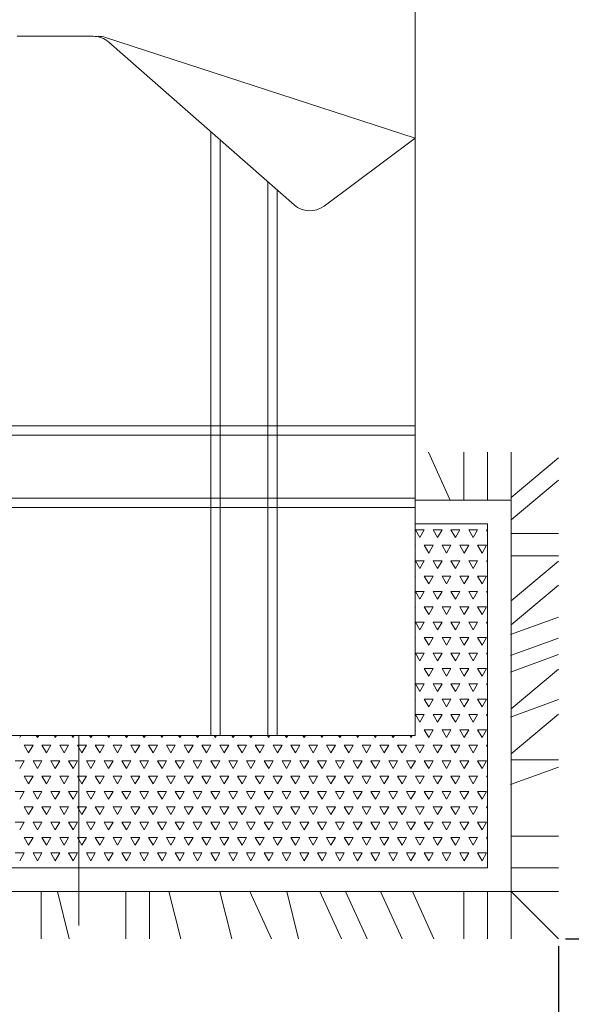
# Model space of a CAD drawing. Units: millimetres. Extents: x 225995 to 227247, y 225507 to 226008.
# Tile 20 of 23: x 227101 to 227150, y 225781 to 225868. Entities that reach past the tile are written whole.
import ezdxf

# ---------------------------------------------------------------- set-up
doc = ezdxf.new("R2010")
doc.units = ezdxf.units.MM
for name, color, linetype, lineweight in [('A-ANNO-DIMS', 2, 'Continuous', 18), ('A-FLOR-PATT', 8, 'Continuous', 13), ('A-FURN', 9, 'Continuous', 18)]:
    doc.layers.add(name, color=color, linetype=linetype, lineweight=lineweight)
doc.styles.get("Standard").update_dxf_attribs({"font": 'arial.ttf'})
doc.dimstyles.new('ISO-25', dxfattribs={"dimtxt": 6, "dimasz": 2.5, "dimexe": 1.25, "dimexo": 0.625, "dimtad": 1, "dimdec": 0, "dimlunit": 3, "dimtxsty": 'Standard', "dimcen": 2.5, "dimadec": 0, "dimazin": 0, "dimtfac": 1, "dimtdec": 0, "dimtmove": 0, "dimatfit": 3, "dimfxl": 1, "dimarcsym": 0})

# ---------------------------------------------------------------- blocks, each defined once
blk = doc.blocks.new('A$C6D2A2628')
for p, q in [((1.791, 2.4297), (1.791, 0.4297)), ((0.9515, 1.9058), (1.1116, 1.9058)), ((1.791, 1.6908), (1.138, 1.9034)), ((1.1446, 1.8934), (1.5358, 1.5497)), ((1.3599, 1.7043), (1.3599, 0.4297)), ((1.3799, 1.6867), (1.3799, 0.4297)), ((1.5987, 1.5472), (1.791, 1.6908)), ((1.4799, 1.5988), (1.4799, 0.4297)), ((1.4999, 1.5812), (1.4999, 0.4297)), ((0.291, 1.0837), (1.791, 1.0837)), ((0.291, 1.0637), (1.791, 1.0637)), ((1.8187, 1.0278), (1.8641, 0.9278)), ((1.8932, 1.0278), (1.8932, 0.9278)), ((1.9432, 1.0278), (1.9432, 0.9278)), ((1.9932, 1.0278), (1.9932, 0.9278)), ((1.9932, 0.9324), (2.0932, 1.016)), ((1.9932, 0.8849), (2.0932, 0.9685)), ((0.291, 0.9307), (1.791, 0.9307)), ((1.9932, 0.9267), (1.791, 0.9267)), ((1.9932, 0.1), (1.9932, 0.9267)), ((0.291, 0.9107), (1.791, 0.9107)), ((1.9432, 0.8767), (1.791, 0.8767)), ((1.9432, 0.15), (1.9432, 0.8767)), ((1.8007, 0.8473), (1.7913, 0.8636)), ((1.7913, 0.8636), (1.8101, 0.8636)), ((1.8007, 0.8473), (1.8101, 0.8636)), ((1.8382, 0.8473), (1.8288, 0.8636)), ((1.8288, 0.8636), (1.8476, 0.8636)), ((1.8382, 0.8473), (1.8476, 0.8636)), ((1.8757, 0.8473), (1.8663, 0.8636)), ((1.8663, 0.8636), (1.8851, 0.8636)), ((1.8757, 0.8473), (1.8851, 0.8636)), ((1.9132, 0.8473), (1.9038, 0.8636)), ((1.9038, 0.8636), (1.9226, 0.8636)), ((1.9132, 0.8473), (1.9226, 0.8636)), ((1.9432, 0.8604), (1.9413, 0.8636)), ((1.9413, 0.8636), (1.9432, 0.8636)), ((1.9932, 0.8564), (2.0932, 0.8564)), ((1.791, 0.8305), (1.7913, 0.8311)), ((1.791, 0.8311), (1.7913, 0.8311)), ((1.8195, 0.8148), (1.8101, 0.8311)), ((1.8101, 0.8311), (1.8288, 0.8311)), ((1.8195, 0.8148), (1.8288, 0.8311)), ((1.857, 0.8148), (1.8476, 0.8311)), ((1.8476, 0.8311), (1.8663, 0.8311)), ((1.857, 0.8148), (1.8663, 0.8311)), ((1.8945, 0.8148), (1.8851, 0.8311)), ((1.8851, 0.8311), (1.9038, 0.8311)), ((1.8945, 0.8148), (1.9038, 0.8311)), ((1.932, 0.8148), (1.9226, 0.8311)), ((1.9226, 0.8311), (1.9413, 0.8311)), ((1.932, 0.8148), (1.9413, 0.8311)), ((1.8007, 0.7824), (1.7913, 0.7986)), ((1.7913, 0.7986), (1.8101, 0.7986)), ((1.8007, 0.7824), (1.8101, 0.7986)), ((1.8382, 0.7824), (1.8288, 0.7986)), ((1.8288, 0.7986), (1.8476, 0.7986)), ((1.8382, 0.7824), (1.8476, 0.7986)), ((1.8757, 0.7824), (1.8663, 0.7986)), ((1.8663, 0.7986), (1.8851, 0.7986)), ((1.8757, 0.7824), (1.8851, 0.7986)), ((1.9132, 0.7824), (1.9038, 0.7986)), ((1.9038, 0.7986), (1.9226, 0.7986)), ((1.9132, 0.7824), (1.9226, 0.7986)), ((1.9432, 0.7955), (1.9413, 0.7986)), ((1.9413, 0.7986), (1.9432, 0.7986)), ((1.9932, 0.8089), (2.0932, 0.8089)), ((1.9932, 0.7139), (2.0932, 0.7975)), ((1.791, 0.7655), (1.7913, 0.7661)), ((1.791, 0.7661), (1.7913, 0.7661)), ((1.8195, 0.7499), (1.8101, 0.7661)), ((1.8101, 0.7661), (1.8288, 0.7661)), ((1.8195, 0.7499), (1.8288, 0.7661)), ((1.857, 0.7499), (1.8476, 0.7661)), ((1.8476, 0.7661), (1.8663, 0.7661)), ((1.857, 0.7499), (1.8663, 0.7661)), ((1.8945, 0.7499), (1.8851, 0.7661)), ((1.8851, 0.7661), (1.9038, 0.7661)), ((1.8945, 0.7499), (1.9038, 0.7661)), ((1.932, 0.7499), (1.9226, 0.7661)), ((1.9226, 0.7661), (1.9413, 0.7661)), ((1.932, 0.7499), (1.9413, 0.7661)), ((1.8007, 0.7174), (1.7913, 0.7337)), ((1.7913, 0.7337), (1.8101, 0.7337)), ((1.8007, 0.7174), (1.8101, 0.7337)), ((1.8382, 0.7174), (1.8288, 0.7337)), ((1.8288, 0.7337), (1.8476, 0.7337)), ((1.8382, 0.7174), (1.8476, 0.7337)), ((1.8757, 0.7174), (1.8663, 0.7337)), ((1.8663, 0.7337), (1.8851, 0.7337)), ((1.8757, 0.7174), (1.8851, 0.7337)), ((1.9132, 0.7174), (1.9038, 0.7337)), ((1.9038, 0.7337), (1.9226, 0.7337)), ((1.9132, 0.7174), (1.9226, 0.7337)), ((1.9432, 0.7305), (1.9413, 0.7337)), ((1.9413, 0.7337), (1.9432, 0.7337)), ((1.9932, 0.6633), (2.0932, 0.7469)), ((1.791, 0.7006), (1.7913, 0.7012)), ((1.791, 0.7012), (1.7913, 0.7012)), ((1.8195, 0.6849), (1.8101, 0.7012)), ((1.8101, 0.7012), (1.8288, 0.7012)), ((1.8195, 0.6849), (1.8288, 0.7012)), ((1.857, 0.6849), (1.8476, 0.7012)), ((1.8476, 0.7012), (1.8663, 0.7012)), ((1.857, 0.6849), (1.8663, 0.7012)), ((1.8945, 0.6849), (1.8851, 0.7012)), ((1.8851, 0.7012), (1.9038, 0.7012)), ((1.8945, 0.6849), (1.9038, 0.7012)), ((1.932, 0.6849), (1.9226, 0.7012)), ((1.9226, 0.7012), (1.9413, 0.7012)), ((1.932, 0.6849), (1.9413, 0.7012)), ((1.8007, 0.6525), (1.7913, 0.6687)), ((1.7913, 0.6687), (1.8101, 0.6687)), ((1.8007, 0.6525), (1.8101, 0.6687)), ((1.8382, 0.6525), (1.8288, 0.6687)), ((1.8288, 0.6687), (1.8476, 0.6687)), ((1.8382, 0.6525), (1.8476, 0.6687)), ((1.8757, 0.6525), (1.8663, 0.6687)), ((1.8663, 0.6687), (1.8851, 0.6687)), ((1.8757, 0.6525), (1.8851, 0.6687)), ((1.9132, 0.6525), (1.9038, 0.6687)), ((1.9038, 0.6687), (1.9226, 0.6687)), ((1.9132, 0.6525), (1.9226, 0.6687)), ((1.9432, 0.6655), (1.9413, 0.6687)), ((1.9413, 0.6687), (1.9432, 0.6687)), ((1.9917, 0.6428), (2.0932, 0.6794)), ((1.791, 0.6356), (1.7913, 0.6362)), ((1.791, 0.6362), (1.7913, 0.6362)), ((1.8195, 0.62), (1.8101, 0.6362)), ((1.8101, 0.6362), (1.8288, 0.6362)), ((1.8195, 0.62), (1.8288, 0.6362)), ((1.857, 0.62), (1.8476, 0.6362)), ((1.8476, 0.6362), (1.8663, 0.6362)), ((1.857, 0.62), (1.8663, 0.6362)), ((1.8945, 0.62), (1.8851, 0.6362)), ((1.8851, 0.6362), (1.9038, 0.6362)), ((1.8945, 0.62), (1.9038, 0.6362)), ((1.932, 0.62), (1.9226, 0.6362)), ((1.9226, 0.6362), (1.9413, 0.6362)), ((1.932, 0.62), (1.9413, 0.6362)), ((1.9917, 0.5984), (2.0932, 0.6351)), ((1.8007, 0.5875), (1.7913, 0.6037)), ((1.7913, 0.6037), (1.8101, 0.6037)), ((1.8007, 0.5875), (1.8101, 0.6037)), ((1.8382, 0.5875), (1.8288, 0.6037)), ((1.8288, 0.6037), (1.8476, 0.6037)), ((1.8382, 0.5875), (1.8476, 0.6037)), ((1.8757, 0.5875), (1.8663, 0.6037)), ((1.8663, 0.6037), (1.8851, 0.6037)), ((1.8757, 0.5875), (1.8851, 0.6037)), ((1.9132, 0.5875), (1.9038, 0.6037)), ((1.9038, 0.6037), (1.9226, 0.6037)), ((1.9132, 0.5875), (1.9226, 0.6037)), ((1.9432, 0.6006), (1.9413, 0.6037)), ((1.9413, 0.6037), (1.9432, 0.6037)), ((1.9917, 0.5636), (2.0932, 0.6003)), ((1.791, 0.5707), (1.7913, 0.5713)), ((1.791, 0.5713), (1.7913, 0.5713)), ((1.8195, 0.555), (1.8101, 0.5713)), ((1.8101, 0.5713), (1.8288, 0.5713)), ((1.8195, 0.555), (1.8288, 0.5713)), ((1.857, 0.555), (1.8476, 0.5713)), ((1.8476, 0.5713), (1.8663, 0.5713)), ((1.857, 0.555), (1.8663, 0.5713)), ((1.8945, 0.555), (1.8851, 0.5713)), ((1.8851, 0.5713), (1.9038, 0.5713)), ((1.8945, 0.555), (1.9038, 0.5713)), ((1.932, 0.555), (1.9226, 0.5713)), ((1.9226, 0.5713), (1.9413, 0.5713)), ((1.932, 0.555), (1.9413, 0.5713)), ((1.9932, 0.4859), (2.0932, 0.5695)), ((1.8007, 0.5226), (1.7913, 0.5388)), ((1.7913, 0.5388), (1.8101, 0.5388)), ((1.8007, 0.5226), (1.8101, 0.5388)), ((1.8382, 0.5226), (1.8288, 0.5388)), ((1.8288, 0.5388), (1.8476, 0.5388)), ((1.8382, 0.5226), (1.8476, 0.5388)), ((1.8757, 0.5226), (1.8663, 0.5388)), ((1.8663, 0.5388), (1.8851, 0.5388)), ((1.8757, 0.5226), (1.8851, 0.5388)), ((1.9132, 0.5226), (1.9038, 0.5388)), ((1.9038, 0.5388), (1.9226, 0.5388)), ((1.9132, 0.5226), (1.9226, 0.5388)), ((1.9432, 0.5356), (1.9413, 0.5388)), ((1.9413, 0.5388), (1.9432, 0.5388)), ((1.791, 0.5057), (1.7913, 0.5063)), ((1.791, 0.5063), (1.7913, 0.5063)), ((1.8195, 0.4901), (1.8101, 0.5063)), ((1.8101, 0.5063), (1.8288, 0.5063)), ((1.8195, 0.4901), (1.8288, 0.5063)), ((1.857, 0.4901), (1.8476, 0.5063)), ((1.8476, 0.5063), (1.8663, 0.5063)), ((1.857, 0.4901), (1.8663, 0.5063)), ((1.8945, 0.4901), (1.8851, 0.5063)), ((1.8851, 0.5063), (1.9038, 0.5063)), ((1.8945, 0.4901), (1.9038, 0.5063)), ((1.932, 0.4901), (1.9226, 0.5063)), ((1.9226, 0.5063), (1.9413, 0.5063)), ((1.932, 0.4901), (1.9413, 0.5063)), ((1.9917, 0.4686), (2.0932, 0.5053)), ((1.8007, 0.4576), (1.7913, 0.4738)), ((1.7913, 0.4738), (1.8101, 0.4738)), ((1.8007, 0.4576), (1.8101, 0.4738)), ((1.8382, 0.4576), (1.8288, 0.4738)), ((1.8288, 0.4738), (1.8476, 0.4738)), ((1.8382, 0.4576), (1.8476, 0.4738)), ((1.8757, 0.4576), (1.8663, 0.4738)), ((1.8663, 0.4738), (1.8851, 0.4738)), ((1.8757, 0.4576), (1.8851, 0.4738)), ((1.9132, 0.4576), (1.9038, 0.4738)), ((1.9038, 0.4738), (1.9226, 0.4738)), ((1.9132, 0.4576), (1.9226, 0.4738)), ((1.9432, 0.4707), (1.9413, 0.4738)), ((1.9413, 0.4738), (1.9432, 0.4738)), ((1.9932, 0.3909), (2.0932, 0.4745)), ((1.791, 0.4408), (1.7913, 0.4414)), ((1.791, 0.4414), (1.7913, 0.4414)), ((1.8195, 0.4251), (1.8101, 0.4414)), ((1.8101, 0.4414), (1.8288, 0.4414)), ((1.8195, 0.4251), (1.8288, 0.4414)), ((1.857, 0.4251), (1.8476, 0.4414)), ((1.8476, 0.4414), (1.8663, 0.4414)), ((1.857, 0.4251), (1.8663, 0.4414)), ((1.8945, 0.4251), (1.8851, 0.4414)), ((1.8851, 0.4414), (1.9038, 0.4414)), ((1.8945, 0.4251), (1.9038, 0.4414)), ((1.932, 0.4251), (1.9226, 0.4414)), ((1.9226, 0.4414), (1.9413, 0.4414)), ((1.932, 0.4251), (1.9413, 0.4414)), ((1.791, 0.4297), (0.291, 0.4297)), ((0.957, 0.4251), (0.9596, 0.4297)), ((0.9945, 0.4251), (0.9918, 0.4297)), ((0.9945, 0.4251), (0.9971, 0.4297)), ((1.032, 0.4251), (1.0293, 0.4297)), ((1.032, 0.4251), (1.0346, 0.4297)), ((1.0695, 0.4251), (1.0668, 0.4297)), ((1.0695, 0.4251), (1.0721, 0.4297)), ((1.107, 0.4251), (1.1043, 0.4297)), ((1.107, 0.4251), (1.1096, 0.4297)), ((1.1445, 0.4251), (1.1418, 0.4297)), ((1.1445, 0.4251), (1.1471, 0.4297)), ((1.182, 0.4251), (1.1793, 0.4297)), ((1.182, 0.4251), (1.1846, 0.4297)), ((1.2195, 0.4251), (1.2168, 0.4297)), ((1.2195, 0.4251), (1.2221, 0.4297)), ((1.257, 0.4251), (1.2543, 0.4297)), ((1.257, 0.4251), (1.2596, 0.4297)), ((1.2945, 0.4251), (1.2918, 0.4297)), ((1.2945, 0.4251), (1.2971, 0.4297)), ((1.332, 0.4251), (1.3293, 0.4297)), ((1.332, 0.4251), (1.3346, 0.4297)), ((1.3695, 0.4251), (1.3668, 0.4297)), ((1.3695, 0.4251), (1.3721, 0.4297)), ((1.407, 0.4251), (1.4043, 0.4297)), ((1.407, 0.4251), (1.4096, 0.4297)), ((1.4445, 0.4251), (1.4418, 0.4297)), ((1.4445, 0.4251), (1.4471, 0.4297)), ((1.482, 0.4251), (1.4793, 0.4297)), ((1.482, 0.4251), (1.4846, 0.4297)), ((1.5195, 0.4251), (1.5168, 0.4297)), ((1.5195, 0.4251), (1.5221, 0.4297)), ((1.557, 0.4251), (1.5543, 0.4297)), ((1.557, 0.4251), (1.5596, 0.4297)), ((1.5945, 0.4251), (1.5918, 0.4297)), ((1.5945, 0.4251), (1.5971, 0.4297)), ((1.632, 0.4251), (1.6293, 0.4297)), ((1.632, 0.4251), (1.6346, 0.4297)), ((1.6695, 0.4251), (1.6668, 0.4297)), ((1.6695, 0.4251), (1.6721, 0.4297)), ((1.707, 0.4251), (1.7043, 0.4297)), ((1.707, 0.4251), (1.7096, 0.4297)), ((1.7445, 0.4251), (1.7418, 0.4297)), ((1.7445, 0.4251), (1.7471, 0.4297)), ((1.782, 0.4251), (1.7793, 0.4297)), ((1.782, 0.4251), (1.7846, 0.4297)), ((0.9757, 0.3927), (0.9663, 0.4089)), ((0.9663, 0.4089), (0.9851, 0.4089)), ((0.9757, 0.3927), (0.9851, 0.4089)), ((1.0132, 0.3927), (1.0038, 0.4089)), ((1.0038, 0.4089), (1.0226, 0.4089)), ((1.0132, 0.3927), (1.0226, 0.4089)), ((1.0507, 0.3927), (1.0413, 0.4089)), ((1.0413, 0.4089), (1.0601, 0.4089)), ((1.0507, 0.3927), (1.0601, 0.4089)), ((1.0882, 0.3927), (1.0788, 0.4089)), ((1.0788, 0.4089), (1.0976, 0.4089)), ((1.0882, 0.3927), (1.0976, 0.4089)), ((1.1257, 0.3927), (1.1163, 0.4089)), ((1.1163, 0.4089), (1.1351, 0.4089)), ((1.1257, 0.3927), (1.1351, 0.4089)), ((1.1632, 0.3927), (1.1538, 0.4089)), ((1.1538, 0.4089), (1.1726, 0.4089)), ((1.1632, 0.3927), (1.1726, 0.4089)), ((1.2007, 0.3927), (1.1913, 0.4089)), ((1.1913, 0.4089), (1.2101, 0.4089)), ((1.2007, 0.3927), (1.2101, 0.4089)), ((1.2382, 0.3927), (1.2288, 0.4089)), ((1.2288, 0.4089), (1.2476, 0.4089)), ((1.2382, 0.3927), (1.2476, 0.4089)), ((1.2757, 0.3927), (1.2663, 0.4089)), ((1.2663, 0.4089), (1.2851, 0.4089)), ((1.2757, 0.3927), (1.2851, 0.4089)), ((1.3132, 0.3927), (1.3038, 0.4089)), ((1.3038, 0.4089), (1.3226, 0.4089)), ((1.3132, 0.3927), (1.3226, 0.4089)), ((1.3507, 0.3927), (1.3413, 0.4089)), ((1.3413, 0.4089), (1.3601, 0.4089)), ((1.3507, 0.3927), (1.3601, 0.4089)), ((1.3882, 0.3927), (1.3788, 0.4089)), ((1.3788, 0.4089), (1.3976, 0.4089)), ((1.3882, 0.3927), (1.3976, 0.4089)), ((1.4257, 0.3927), (1.4163, 0.4089)), ((1.4163, 0.4089), (1.4351, 0.4089)), ((1.4257, 0.3927), (1.4351, 0.4089)), ((1.4632, 0.3927), (1.4538, 0.4089)), ((1.4538, 0.4089), (1.4726, 0.4089)), ((1.4632, 0.3927), (1.4726, 0.4089)), ((1.5007, 0.3927), (1.4913, 0.4089)), ((1.4913, 0.4089), (1.5101, 0.4089)), ((1.5007, 0.3927), (1.5101, 0.4089)), ((1.5382, 0.3927), (1.5288, 0.4089)), ((1.5288, 0.4089), (1.5476, 0.4089)), ((1.5382, 0.3927), (1.5476, 0.4089)), ((1.5757, 0.3927), (1.5663, 0.4089)), ((1.5663, 0.4089), (1.5851, 0.4089)), ((1.5757, 0.3927), (1.5851, 0.4089)), ((1.6132, 0.3927), (1.6038, 0.4089)), ((1.6038, 0.4089), (1.6226, 0.4089)), ((1.6132, 0.3927), (1.6226, 0.4089)), ((1.6507, 0.3927), (1.6413, 0.4089)), ((1.6413, 0.4089), (1.6601, 0.4089)), ((1.6507, 0.3927), (1.6601, 0.4089)), ((1.6882, 0.3927), (1.6788, 0.4089)), ((1.6788, 0.4089), (1.6976, 0.4089)), ((1.6882, 0.3927), (1.6976, 0.4089)), ((1.7257, 0.3927), (1.7163, 0.4089)), ((1.7163, 0.4089), (1.7351, 0.4089)), ((1.7257, 0.3927), (1.7351, 0.4089)), ((1.7632, 0.3927), (1.7538, 0.4089)), ((1.7538, 0.4089), (1.7726, 0.4089)), ((1.7632, 0.3927), (1.7726, 0.4089)), ((1.8007, 0.3927), (1.7913, 0.4089)), ((1.7913, 0.4089), (1.8101, 0.4089)), ((1.8007, 0.3927), (1.8101, 0.4089)), ((1.8382, 0.3927), (1.8288, 0.4089)), ((1.8288, 0.4089), (1.8476, 0.4089)), ((1.8382, 0.3927), (1.8476, 0.4089)), ((1.8757, 0.3927), (1.8663, 0.4089)), ((1.8663, 0.4089), (1.8851, 0.4089)), ((1.8757, 0.3927), (1.8851, 0.4089)), ((1.9132, 0.3927), (1.9038, 0.4089)), ((1.9038, 0.4089), (1.9226, 0.4089)), ((1.9132, 0.3927), (1.9226, 0.4089)), ((1.9432, 0.4057), (1.9413, 0.4089)), ((1.9413, 0.4089), (1.9432, 0.4089)), ((0.9476, 0.3764), (0.9663, 0.3764)), ((0.957, 0.3602), (0.9663, 0.3764)), ((0.9945, 0.3602), (0.9851, 0.3764)), ((0.9851, 0.3764), (1.0038, 0.3764)), ((0.9945, 0.3602), (1.0038, 0.3764)), ((1.032, 0.3602), (1.0226, 0.3764)), ((1.0226, 0.3764), (1.0413, 0.3764)), ((1.032, 0.3602), (1.0413, 0.3764)), ((1.0695, 0.3602), (1.0601, 0.3764)), ((1.0601, 0.3764), (1.0788, 0.3764)), ((1.0695, 0.3602), (1.0788, 0.3764)), ((1.107, 0.3602), (1.0976, 0.3764)), ((1.0976, 0.3764), (1.1163, 0.3764)), ((1.107, 0.3602), (1.1163, 0.3764)), ((1.1445, 0.3602), (1.1351, 0.3764)), ((1.1351, 0.3764), (1.1538, 0.3764)), ((1.1445, 0.3602), (1.1538, 0.3764)), ((1.182, 0.3602), (1.1726, 0.3764)), ((1.1726, 0.3764), (1.1913, 0.3764)), ((1.182, 0.3602), (1.1913, 0.3764)), ((1.2195, 0.3602), (1.2101, 0.3764)), ((1.2101, 0.3764), (1.2288, 0.3764)), ((1.2195, 0.3602), (1.2288, 0.3764)), ((1.257, 0.3602), (1.2476, 0.3764)), ((1.2476, 0.3764), (1.2663, 0.3764)), ((1.257, 0.3602), (1.2663, 0.3764)), ((1.2945, 0.3602), (1.2851, 0.3764)), ((1.2851, 0.3764), (1.3038, 0.3764)), ((1.2945, 0.3602), (1.3038, 0.3764)), ((1.332, 0.3602), (1.3226, 0.3764)), ((1.3226, 0.3764), (1.3413, 0.3764)), ((1.332, 0.3602), (1.3413, 0.3764)), ((1.3695, 0.3602), (1.3601, 0.3764)), ((1.3601, 0.3764), (1.3788, 0.3764)), ((1.3695, 0.3602), (1.3788, 0.3764)), ((1.407, 0.3602), (1.3976, 0.3764)), ((1.3976, 0.3764), (1.4163, 0.3764)), ((1.407, 0.3602), (1.4163, 0.3764)), ((1.4445, 0.3602), (1.4351, 0.3764)), ((1.4351, 0.3764), (1.4538, 0.3764)), ((1.4445, 0.3602), (1.4538, 0.3764)), ((1.482, 0.3602), (1.4726, 0.3764)), ((1.4726, 0.3764), (1.4913, 0.3764)), ((1.482, 0.3602), (1.4913, 0.3764)), ((1.5195, 0.3602), (1.5101, 0.3764)), ((1.5101, 0.3764), (1.5288, 0.3764)), ((1.5195, 0.3602), (1.5288, 0.3764)), ((1.557, 0.3602), (1.5476, 0.3764)), ((1.5476, 0.3764), (1.5663, 0.3764)), ((1.557, 0.3602), (1.5663, 0.3764)), ((1.5945, 0.3602), (1.5851, 0.3764)), ((1.5851, 0.3764), (1.6038, 0.3764)), ((1.5945, 0.3602), (1.6038, 0.3764)), ((1.632, 0.3602), (1.6226, 0.3764)), ((1.6226, 0.3764), (1.6413, 0.3764)), ((1.632, 0.3602), (1.6413, 0.3764)), ((1.6695, 0.3602), (1.6601, 0.3764)), ((1.6601, 0.3764), (1.6788, 0.3764)), ((1.6695, 0.3602), (1.6788, 0.3764)), ((1.707, 0.3602), (1.6976, 0.3764)), ((1.6976, 0.3764), (1.7163, 0.3764)), ((1.707, 0.3602), (1.7163, 0.3764)), ((1.7445, 0.3602), (1.7351, 0.3764)), ((1.7351, 0.3764), (1.7538, 0.3764)), ((1.7445, 0.3602), (1.7538, 0.3764)), ((1.782, 0.3602), (1.7726, 0.3764)), ((1.7726, 0.3764), (1.7913, 0.3764)), ((1.782, 0.3602), (1.7913, 0.3764)), ((1.8195, 0.3602), (1.8101, 0.3764)), ((1.8101, 0.3764), (1.8288, 0.3764)), ((1.8195, 0.3602), (1.8288, 0.3764)), ((1.857, 0.3602), (1.8476, 0.3764)), ((1.8476, 0.3764), (1.8663, 0.3764)), ((1.857, 0.3602), (1.8663, 0.3764)), ((1.8945, 0.3602), (1.8851, 0.3764)), ((1.8851, 0.3764), (1.9038, 0.3764)), ((1.8945, 0.3602), (1.9038, 0.3764)), ((1.932, 0.3602), (1.9226, 0.3764)), ((1.9226, 0.3764), (1.9413, 0.3764)), ((1.932, 0.3602), (1.9413, 0.3764)), ((1.9932, 0.3783), (2.0932, 0.3783)), ((1.9917, 0.3261), (2.0932, 0.3628)), ((0.9757, 0.3277), (0.9663, 0.3439)), ((0.9663, 0.3439), (0.9851, 0.3439)), ((0.9757, 0.3277), (0.9851, 0.3439)), ((1.0132, 0.3277), (1.0038, 0.3439)), ((1.0038, 0.3439), (1.0226, 0.3439)), ((1.0132, 0.3277), (1.0226, 0.3439)), ((1.0507, 0.3277), (1.0413, 0.3439)), ((1.0413, 0.3439), (1.0601, 0.3439)), ((1.0507, 0.3277), (1.0601, 0.3439)), ((1.0882, 0.3277), (1.0788, 0.3439)), ((1.0788, 0.3439), (1.0976, 0.3439)), ((1.0882, 0.3277), (1.0976, 0.3439)), ((1.1257, 0.3277), (1.1163, 0.3439)), ((1.1163, 0.3439), (1.1351, 0.3439)), ((1.1257, 0.3277), (1.1351, 0.3439)), ((1.1632, 0.3277), (1.1538, 0.3439)), ((1.1538, 0.3439), (1.1726, 0.3439)), ((1.1632, 0.3277), (1.1726, 0.3439)), ((1.2007, 0.3277), (1.1913, 0.3439)), ((1.1913, 0.3439), (1.2101, 0.3439)), ((1.2007, 0.3277), (1.2101, 0.3439)), ((1.2382, 0.3277), (1.2288, 0.3439)), ((1.2288, 0.3439), (1.2476, 0.3439)), ((1.2382, 0.3277), (1.2476, 0.3439)), ((1.2757, 0.3277), (1.2663, 0.3439)), ((1.2663, 0.3439), (1.2851, 0.3439)), ((1.2757, 0.3277), (1.2851, 0.3439)), ((1.3132, 0.3277), (1.3038, 0.3439)), ((1.3038, 0.3439), (1.3226, 0.3439)), ((1.3132, 0.3277), (1.3226, 0.3439)), ((1.3507, 0.3277), (1.3413, 0.3439)), ((1.3413, 0.3439), (1.3601, 0.3439)), ((1.3507, 0.3277), (1.3601, 0.3439)), ((1.3882, 0.3277), (1.3788, 0.3439)), ((1.3788, 0.3439), (1.3976, 0.3439)), ((1.3882, 0.3277), (1.3976, 0.3439)), ((1.4257, 0.3277), (1.4163, 0.3439)), ((1.4163, 0.3439), (1.4351, 0.3439)), ((1.4257, 0.3277), (1.4351, 0.3439)), ((1.4632, 0.3277), (1.4538, 0.3439)), ((1.4538, 0.3439), (1.4726, 0.3439)), ((1.4632, 0.3277), (1.4726, 0.3439)), ((1.5007, 0.3277), (1.4913, 0.3439)), ((1.4913, 0.3439), (1.5101, 0.3439)), ((1.5007, 0.3277), (1.5101, 0.3439)), ((1.5382, 0.3277), (1.5288, 0.3439)), ((1.5288, 0.3439), (1.5476, 0.3439)), ((1.5382, 0.3277), (1.5476, 0.3439)), ((1.5757, 0.3277), (1.5663, 0.3439)), ((1.5663, 0.3439), (1.5851, 0.3439)), ((1.5757, 0.3277), (1.5851, 0.3439)), ((1.6132, 0.3277), (1.6038, 0.3439)), ((1.6038, 0.3439), (1.6226, 0.3439)), ((1.6132, 0.3277), (1.6226, 0.3439)), ((1.6507, 0.3277), (1.6413, 0.3439)), ((1.6413, 0.3439), (1.6601, 0.3439)), ((1.6507, 0.3277), (1.6601, 0.3439)), ((1.6882, 0.3277), (1.6788, 0.3439)), ((1.6788, 0.3439), (1.6976, 0.3439)), ((1.6882, 0.3277), (1.6976, 0.3439)), ((1.7257, 0.3277), (1.7163, 0.3439)), ((1.7163, 0.3439), (1.7351, 0.3439)), ((1.7257, 0.3277), (1.7351, 0.3439)), ((1.7632, 0.3277), (1.7538, 0.3439)), ((1.7538, 0.3439), (1.7726, 0.3439)), ((1.7632, 0.3277), (1.7726, 0.3439)), ((1.8007, 0.3277), (1.7913, 0.3439)), ((1.7913, 0.3439), (1.8101, 0.3439)), ((1.8007, 0.3277), (1.8101, 0.3439)), ((1.8382, 0.3277), (1.8288, 0.3439)), ((1.8288, 0.3439), (1.8476, 0.3439)), ((1.8382, 0.3277), (1.8476, 0.3439)), ((1.8757, 0.3277), (1.8663, 0.3439)), ((1.8663, 0.3439), (1.8851, 0.3439)), ((1.8757, 0.3277), (1.8851, 0.3439)), ((1.9132, 0.3277), (1.9038, 0.3439)), ((1.9038, 0.3439), (1.9226, 0.3439)), ((1.9132, 0.3277), (1.9226, 0.3439)), ((1.9432, 0.3408), (1.9413, 0.3439)), ((1.9413, 0.3439), (1.9432, 0.3439)), ((0.9476, 0.3115), (0.9663, 0.3115)), ((0.957, 0.2952), (0.9663, 0.3115)), ((0.9945, 0.2952), (0.9851, 0.3115)), ((0.9851, 0.3115), (1.0038, 0.3115)), ((0.9945, 0.2952), (1.0038, 0.3115)), ((1.032, 0.2952), (1.0226, 0.3115)), ((1.0226, 0.3115), (1.0413, 0.3115)), ((1.032, 0.2952), (1.0413, 0.3115)), ((1.0695, 0.2952), (1.0601, 0.3115)), ((1.0601, 0.3115), (1.0788, 0.3115)), ((1.0695, 0.2952), (1.0788, 0.3115)), ((1.107, 0.2952), (1.0976, 0.3115)), ((1.0976, 0.3115), (1.1163, 0.3115)), ((1.107, 0.2952), (1.1163, 0.3115)), ((1.1445, 0.2952), (1.1351, 0.3115)), ((1.1351, 0.3115), (1.1538, 0.3115)), ((1.1445, 0.2952), (1.1538, 0.3115)), ((1.182, 0.2952), (1.1726, 0.3115)), ((1.1726, 0.3115), (1.1913, 0.3115)), ((1.182, 0.2952), (1.1913, 0.3115)), ((1.2195, 0.2952), (1.2101, 0.3115)), ((1.2101, 0.3115), (1.2288, 0.3115)), ((1.2195, 0.2952), (1.2288, 0.3115)), ((1.257, 0.2952), (1.2476, 0.3115)), ((1.2476, 0.3115), (1.2663, 0.3115)), ((1.257, 0.2952), (1.2663, 0.3115)), ((1.2945, 0.2952), (1.2851, 0.3115)), ((1.2851, 0.3115), (1.3038, 0.3115)), ((1.2945, 0.2952), (1.3038, 0.3115)), ((1.332, 0.2952), (1.3226, 0.3115)), ((1.3226, 0.3115), (1.3413, 0.3115)), ((1.332, 0.2952), (1.3413, 0.3115)), ((1.3695, 0.2952), (1.3601, 0.3115)), ((1.3601, 0.3115), (1.3788, 0.3115)), ((1.3695, 0.2952), (1.3788, 0.3115)), ((1.407, 0.2952), (1.3976, 0.3115)), ((1.3976, 0.3115), (1.4163, 0.3115)), ((1.407, 0.2952), (1.4163, 0.3115)), ((1.4445, 0.2952), (1.4351, 0.3115)), ((1.4351, 0.3115), (1.4538, 0.3115)), ((1.4445, 0.2952), (1.4538, 0.3115)), ((1.482, 0.2952), (1.4726, 0.3115)), ((1.4726, 0.3115), (1.4913, 0.3115)), ((1.482, 0.2952), (1.4913, 0.3115)), ((1.5195, 0.2952), (1.5101, 0.3115)), ((1.5101, 0.3115), (1.5288, 0.3115)), ((1.5195, 0.2952), (1.5288, 0.3115)), ((1.557, 0.2952), (1.5476, 0.3115)), ((1.5476, 0.3115), (1.5663, 0.3115)), ((1.557, 0.2952), (1.5663, 0.3115)), ((1.5945, 0.2952), (1.5851, 0.3115)), ((1.5851, 0.3115), (1.6038, 0.3115)), ((1.5945, 0.2952), (1.6038, 0.3115)), ((1.632, 0.2952), (1.6226, 0.3115)), ((1.6226, 0.3115), (1.6413, 0.3115)), ((1.632, 0.2952), (1.6413, 0.3115)), ((1.6695, 0.2952), (1.6601, 0.3115)), ((1.6601, 0.3115), (1.6788, 0.3115)), ((1.6695, 0.2952), (1.6788, 0.3115)), ((1.707, 0.2952), (1.6976, 0.3115)), ((1.6976, 0.3115), (1.7163, 0.3115)), ((1.707, 0.2952), (1.7163, 0.3115)), ((1.7445, 0.2952), (1.7351, 0.3115)), ((1.7351, 0.3115), (1.7538, 0.3115)), ((1.7445, 0.2952), (1.7538, 0.3115)), ((1.782, 0.2952), (1.7726, 0.3115)), ((1.7726, 0.3115), (1.7913, 0.3115)), ((1.782, 0.2952), (1.7913, 0.3115)), ((1.8195, 0.2952), (1.8101, 0.3115)), ((1.8101, 0.3115), (1.8288, 0.3115)), ((1.8195, 0.2952), (1.8288, 0.3115)), ((1.857, 0.2952), (1.8476, 0.3115)), ((1.8476, 0.3115), (1.8663, 0.3115)), ((1.857, 0.2952), (1.8663, 0.3115)), ((1.8945, 0.2952), (1.8851, 0.3115)), ((1.8851, 0.3115), (1.9038, 0.3115)), ((1.8945, 0.2952), (1.9038, 0.3115)), ((1.932, 0.2952), (1.9226, 0.3115)), ((1.9226, 0.3115), (1.9413, 0.3115)), ((1.932, 0.2952), (1.9413, 0.3115)), ((0.9757, 0.2628), (0.9663, 0.279)), ((0.9663, 0.279), (0.9851, 0.279)), ((0.9757, 0.2628), (0.9851, 0.279)), ((1.0132, 0.2628), (1.0038, 0.279)), ((1.0038, 0.279), (1.0226, 0.279)), ((1.0132, 0.2628), (1.0226, 0.279)), ((1.0507, 0.2628), (1.0413, 0.279)), ((1.0413, 0.279), (1.0601, 0.279)), ((1.0507, 0.2628), (1.0601, 0.279)), ((1.0882, 0.2628), (1.0788, 0.279)), ((1.0788, 0.279), (1.0976, 0.279)), ((1.0882, 0.2628), (1.0976, 0.279)), ((1.1257, 0.2628), (1.1163, 0.279)), ((1.1163, 0.279), (1.1351, 0.279)), ((1.1257, 0.2628), (1.1351, 0.279)), ((1.1632, 0.2628), (1.1538, 0.279)), ((1.1538, 0.279), (1.1726, 0.279)), ((1.1632, 0.2628), (1.1726, 0.279)), ((1.2007, 0.2628), (1.1913, 0.279)), ((1.1913, 0.279), (1.2101, 0.279)), ((1.2007, 0.2628), (1.2101, 0.279)), ((1.2382, 0.2628), (1.2288, 0.279)), ((1.2288, 0.279), (1.2476, 0.279)), ((1.2382, 0.2628), (1.2476, 0.279)), ((1.2757, 0.2628), (1.2663, 0.279)), ((1.2663, 0.279), (1.2851, 0.279)), ((1.2757, 0.2628), (1.2851, 0.279)), ((1.3132, 0.2628), (1.3038, 0.279)), ((1.3038, 0.279), (1.3226, 0.279)), ((1.3132, 0.2628), (1.3226, 0.279)), ((1.3507, 0.2628), (1.3413, 0.279)), ((1.3413, 0.279), (1.3601, 0.279)), ((1.3507, 0.2628), (1.3601, 0.279)), ((1.3882, 0.2628), (1.3788, 0.279)), ((1.3788, 0.279), (1.3976, 0.279)), ((1.3882, 0.2628), (1.3976, 0.279)), ((1.4257, 0.2628), (1.4163, 0.279)), ((1.4163, 0.279), (1.4351, 0.279)), ((1.4257, 0.2628), (1.4351, 0.279)), ((1.4632, 0.2628), (1.4538, 0.279)), ((1.4538, 0.279), (1.4726, 0.279)), ((1.4632, 0.2628), (1.4726, 0.279)), ((1.5007, 0.2628), (1.4913, 0.279)), ((1.4913, 0.279), (1.5101, 0.279)), ((1.5007, 0.2628), (1.5101, 0.279)), ((1.5382, 0.2628), (1.5288, 0.279)), ((1.5288, 0.279), (1.5476, 0.279)), ((1.5382, 0.2628), (1.5476, 0.279)), ((1.5757, 0.2628), (1.5663, 0.279)), ((1.5663, 0.279), (1.5851, 0.279)), ((1.5757, 0.2628), (1.5851, 0.279)), ((1.6132, 0.2628), (1.6038, 0.279)), ((1.6038, 0.279), (1.6226, 0.279)), ((1.6132, 0.2628), (1.6226, 0.279)), ((1.6507, 0.2628), (1.6413, 0.279)), ((1.6413, 0.279), (1.6601, 0.279)), ((1.6507, 0.2628), (1.6601, 0.279)), ((1.6882, 0.2628), (1.6788, 0.279)), ((1.6788, 0.279), (1.6976, 0.279)), ((1.6882, 0.2628), (1.6976, 0.279)), ((1.7257, 0.2628), (1.7163, 0.279)), ((1.7163, 0.279), (1.7351, 0.279)), ((1.7257, 0.2628), (1.7351, 0.279)), ((1.7632, 0.2628), (1.7538, 0.279)), ((1.7538, 0.279), (1.7726, 0.279)), ((1.7632, 0.2628), (1.7726, 0.279)), ((1.8007, 0.2628), (1.7913, 0.279)), ((1.7913, 0.279), (1.8101, 0.279)), ((1.8007, 0.2628), (1.8101, 0.279)), ((1.8382, 0.2628), (1.8288, 0.279)), ((1.8288, 0.279), (1.8476, 0.279)), ((1.8382, 0.2628), (1.8476, 0.279)), ((1.8757, 0.2628), (1.8663, 0.279)), ((1.8663, 0.279), (1.8851, 0.279)), ((1.8757, 0.2628), (1.8851, 0.279)), ((1.9132, 0.2628), (1.9038, 0.279)), ((1.9038, 0.279), (1.9226, 0.279)), ((1.9132, 0.2628), (1.9226, 0.279)), ((1.9432, 0.2758), (1.9413, 0.279)), ((1.9413, 0.279), (1.9432, 0.279)), ((0.9476, 0.2465), (0.9663, 0.2465)), ((0.957, 0.2303), (0.9663, 0.2465)), ((0.9945, 0.2303), (0.9851, 0.2465)), ((0.9851, 0.2465), (1.0038, 0.2465)), ((0.9945, 0.2303), (1.0038, 0.2465)), ((1.032, 0.2303), (1.0226, 0.2465)), ((1.0226, 0.2465), (1.0413, 0.2465)), ((1.032, 0.2303), (1.0413, 0.2465)), ((1.0695, 0.2303), (1.0601, 0.2465)), ((1.0601, 0.2465), (1.0788, 0.2465)), ((1.0695, 0.2303), (1.0788, 0.2465)), ((1.107, 0.2303), (1.0976, 0.2465)), ((1.0976, 0.2465), (1.1163, 0.2465)), ((1.107, 0.2303), (1.1163, 0.2465)), ((1.1445, 0.2303), (1.1351, 0.2465)), ((1.1351, 0.2465), (1.1538, 0.2465)), ((1.1445, 0.2303), (1.1538, 0.2465)), ((1.182, 0.2303), (1.1726, 0.2465)), ((1.1726, 0.2465), (1.1913, 0.2465)), ((1.182, 0.2303), (1.1913, 0.2465)), ((1.2195, 0.2303), (1.2101, 0.2465)), ((1.2101, 0.2465), (1.2288, 0.2465)), ((1.2195, 0.2303), (1.2288, 0.2465)), ((1.257, 0.2303), (1.2476, 0.2465)), ((1.2476, 0.2465), (1.2663, 0.2465)), ((1.257, 0.2303), (1.2663, 0.2465)), ((1.2945, 0.2303), (1.2851, 0.2465)), ((1.2851, 0.2465), (1.3038, 0.2465)), ((1.2945, 0.2303), (1.3038, 0.2465)), ((1.332, 0.2303), (1.3226, 0.2465)), ((1.3226, 0.2465), (1.3413, 0.2465)), ((1.332, 0.2303), (1.3413, 0.2465)), ((1.3695, 0.2303), (1.3601, 0.2465)), ((1.3601, 0.2465), (1.3788, 0.2465)), ((1.3695, 0.2303), (1.3788, 0.2465)), ((1.407, 0.2303), (1.3976, 0.2465)), ((1.3976, 0.2465), (1.4163, 0.2465)), ((1.407, 0.2303), (1.4163, 0.2465)), ((1.4445, 0.2303), (1.4351, 0.2465)), ((1.4351, 0.2465), (1.4538, 0.2465)), ((1.4445, 0.2303), (1.4538, 0.2465)), ((1.482, 0.2303), (1.4726, 0.2465)), ((1.4726, 0.2465), (1.4913, 0.2465)), ((1.482, 0.2303), (1.4913, 0.2465)), ((1.5195, 0.2303), (1.5101, 0.2465)), ((1.5101, 0.2465), (1.5288, 0.2465)), ((1.5195, 0.2303), (1.5288, 0.2465)), ((1.557, 0.2303), (1.5476, 0.2465)), ((1.5476, 0.2465), (1.5663, 0.2465)), ((1.557, 0.2303), (1.5663, 0.2465)), ((1.5945, 0.2303), (1.5851, 0.2465)), ((1.5851, 0.2465), (1.6038, 0.2465)), ((1.5945, 0.2303), (1.6038, 0.2465)), ((1.632, 0.2303), (1.6226, 0.2465)), ((1.6226, 0.2465), (1.6413, 0.2465)), ((1.632, 0.2303), (1.6413, 0.2465)), ((1.6695, 0.2303), (1.6601, 0.2465)), ((1.6601, 0.2465), (1.6788, 0.2465)), ((1.6695, 0.2303), (1.6788, 0.2465)), ((1.707, 0.2303), (1.6976, 0.2465)), ((1.6976, 0.2465), (1.7163, 0.2465)), ((1.707, 0.2303), (1.7163, 0.2465)), ((1.7445, 0.2303), (1.7351, 0.2465)), ((1.7351, 0.2465), (1.7538, 0.2465)), ((1.7445, 0.2303), (1.7538, 0.2465)), ((1.782, 0.2303), (1.7726, 0.2465)), ((1.7726, 0.2465), (1.7913, 0.2465)), ((1.782, 0.2303), (1.7913, 0.2465)), ((1.8195, 0.2303), (1.8101, 0.2465)), ((1.8101, 0.2465), (1.8288, 0.2465)), ((1.8195, 0.2303), (1.8288, 0.2465)), ((1.857, 0.2303), (1.8476, 0.2465)), ((1.8476, 0.2465), (1.8663, 0.2465)), ((1.857, 0.2303), (1.8663, 0.2465)), ((1.8945, 0.2303), (1.8851, 0.2465)), ((1.8851, 0.2465), (1.9038, 0.2465)), ((1.8945, 0.2303), (1.9038, 0.2465)), ((1.932, 0.2303), (1.9226, 0.2465)), ((1.9226, 0.2465), (1.9413, 0.2465)), ((1.932, 0.2303), (1.9413, 0.2465)), ((0.9757, 0.1978), (0.9663, 0.214)), ((0.9663, 0.214), (0.9851, 0.214)), ((0.9757, 0.1978), (0.9851, 0.214)), ((1.0132, 0.1978), (1.0038, 0.214)), ((1.0038, 0.214), (1.0226, 0.214)), ((1.0132, 0.1978), (1.0226, 0.214)), ((1.0507, 0.1978), (1.0413, 0.214)), ((1.0413, 0.214), (1.0601, 0.214)), ((1.0507, 0.1978), (1.0601, 0.214)), ((1.0882, 0.1978), (1.0788, 0.214)), ((1.0788, 0.214), (1.0976, 0.214)), ((1.0882, 0.1978), (1.0976, 0.214)), ((1.1257, 0.1978), (1.1163, 0.214)), ((1.1163, 0.214), (1.1351, 0.214)), ((1.1257, 0.1978), (1.1351, 0.214)), ((1.1632, 0.1978), (1.1538, 0.214)), ((1.1538, 0.214), (1.1726, 0.214)), ((1.1632, 0.1978), (1.1726, 0.214)), ((1.2007, 0.1978), (1.1913, 0.214)), ((1.1913, 0.214), (1.2101, 0.214)), ((1.2007, 0.1978), (1.2101, 0.214)), ((1.2382, 0.1978), (1.2288, 0.214)), ((1.2288, 0.214), (1.2476, 0.214)), ((1.2382, 0.1978), (1.2476, 0.214)), ((1.2757, 0.1978), (1.2663, 0.214)), ((1.2663, 0.214), (1.2851, 0.214)), ((1.2757, 0.1978), (1.2851, 0.214)), ((1.3132, 0.1978), (1.3038, 0.214)), ((1.3038, 0.214), (1.3226, 0.214)), ((1.3132, 0.1978), (1.3226, 0.214)), ((1.3507, 0.1978), (1.3413, 0.214)), ((1.3413, 0.214), (1.3601, 0.214)), ((1.3507, 0.1978), (1.3601, 0.214)), ((1.3882, 0.1978), (1.3788, 0.214)), ((1.3788, 0.214), (1.3976, 0.214)), ((1.3882, 0.1978), (1.3976, 0.214)), ((1.4257, 0.1978), (1.4163, 0.214)), ((1.4163, 0.214), (1.4351, 0.214)), ((1.4257, 0.1978), (1.4351, 0.214)), ((1.4632, 0.1978), (1.4538, 0.214)), ((1.4538, 0.214), (1.4726, 0.214)), ((1.4632, 0.1978), (1.4726, 0.214)), ((1.5007, 0.1978), (1.4913, 0.214)), ((1.4913, 0.214), (1.5101, 0.214)), ((1.5007, 0.1978), (1.5101, 0.214)), ((1.5382, 0.1978), (1.5288, 0.214)), ((1.5288, 0.214), (1.5476, 0.214)), ((1.5382, 0.1978), (1.5476, 0.214)), ((1.5757, 0.1978), (1.5663, 0.214)), ((1.5663, 0.214), (1.5851, 0.214)), ((1.5757, 0.1978), (1.5851, 0.214)), ((1.6132, 0.1978), (1.6038, 0.214)), ((1.6038, 0.214), (1.6226, 0.214)), ((1.6132, 0.1978), (1.6226, 0.214)), ((1.6507, 0.1978), (1.6413, 0.214)), ((1.6413, 0.214), (1.6601, 0.214)), ((1.6507, 0.1978), (1.6601, 0.214)), ((1.6882, 0.1978), (1.6788, 0.214)), ((1.6788, 0.214), (1.6976, 0.214)), ((1.6882, 0.1978), (1.6976, 0.214)), ((1.7257, 0.1978), (1.7163, 0.214)), ((1.7163, 0.214), (1.7351, 0.214)), ((1.7257, 0.1978), (1.7351, 0.214)), ((1.7632, 0.1978), (1.7538, 0.214)), ((1.7538, 0.214), (1.7726, 0.214)), ((1.7632, 0.1978), (1.7726, 0.214)), ((1.8007, 0.1978), (1.7913, 0.214)), ((1.7913, 0.214), (1.8101, 0.214)), ((1.8007, 0.1978), (1.8101, 0.214)), ((1.8382, 0.1978), (1.8288, 0.214)), ((1.8288, 0.214), (1.8476, 0.214)), ((1.8382, 0.1978), (1.8476, 0.214)), ((1.8757, 0.1978), (1.8663, 0.214)), ((1.8663, 0.214), (1.8851, 0.214)), ((1.8757, 0.1978), (1.8851, 0.214)), ((1.9132, 0.1978), (1.9038, 0.214)), ((1.9038, 0.214), (1.9226, 0.214)), ((1.9132, 0.1978), (1.9226, 0.214)), ((1.9432, 0.2109), (1.9413, 0.214)), ((1.9413, 0.214), (1.9432, 0.214)), ((1.9932, 0.2173), (2.0932, 0.2173)), ((0.9476, 0.1816), (0.9663, 0.1816)), ((0.957, 0.1653), (0.9663, 0.1816)), ((0.9945, 0.1653), (0.9851, 0.1816)), ((0.9851, 0.1816), (1.0038, 0.1816)), ((0.9945, 0.1653), (1.0038, 0.1816)), ((1.032, 0.1653), (1.0226, 0.1816)), ((1.0226, 0.1816), (1.0413, 0.1816)), ((1.032, 0.1653), (1.0413, 0.1816)), ((1.0695, 0.1653), (1.0601, 0.1816)), ((1.0601, 0.1816), (1.0788, 0.1816)), ((1.0695, 0.1653), (1.0788, 0.1816)), ((1.107, 0.1653), (1.0976, 0.1816)), ((1.0976, 0.1816), (1.1163, 0.1816)), ((1.107, 0.1653), (1.1163, 0.1816)), ((1.1445, 0.1653), (1.1351, 0.1816)), ((1.1351, 0.1816), (1.1538, 0.1816)), ((1.1445, 0.1653), (1.1538, 0.1816)), ((1.182, 0.1653), (1.1726, 0.1816)), ((1.1726, 0.1816), (1.1913, 0.1816)), ((1.182, 0.1653), (1.1913, 0.1816)), ((1.2195, 0.1653), (1.2101, 0.1816)), ((1.2101, 0.1816), (1.2288, 0.1816)), ((1.2195, 0.1653), (1.2288, 0.1816)), ((1.257, 0.1653), (1.2476, 0.1816)), ((1.2476, 0.1816), (1.2663, 0.1816)), ((1.257, 0.1653), (1.2663, 0.1816)), ((1.2945, 0.1653), (1.2851, 0.1816)), ((1.2851, 0.1816), (1.3038, 0.1816)), ((1.2945, 0.1653), (1.3038, 0.1816)), ((1.332, 0.1653), (1.3226, 0.1816)), ((1.3226, 0.1816), (1.3413, 0.1816)), ((1.332, 0.1653), (1.3413, 0.1816)), ((1.3695, 0.1653), (1.3601, 0.1816)), ((1.3601, 0.1816), (1.3788, 0.1816)), ((1.3695, 0.1653), (1.3788, 0.1816)), ((1.407, 0.1653), (1.3976, 0.1816)), ((1.3976, 0.1816), (1.4163, 0.1816)), ((1.407, 0.1653), (1.4163, 0.1816)), ((1.4445, 0.1653), (1.4351, 0.1816)), ((1.4351, 0.1816), (1.4538, 0.1816)), ((1.4445, 0.1653), (1.4538, 0.1816)), ((1.482, 0.1653), (1.4726, 0.1816)), ((1.4726, 0.1816), (1.4913, 0.1816)), ((1.482, 0.1653), (1.4913, 0.1816)), ((1.5195, 0.1653), (1.5101, 0.1816)), ((1.5101, 0.1816), (1.5288, 0.1816)), ((1.5195, 0.1653), (1.5288, 0.1816)), ((1.557, 0.1653), (1.5476, 0.1816)), ((1.5476, 0.1816), (1.5663, 0.1816)), ((1.557, 0.1653), (1.5663, 0.1816)), ((1.5945, 0.1653), (1.5851, 0.1816)), ((1.5851, 0.1816), (1.6038, 0.1816)), ((1.5945, 0.1653), (1.6038, 0.1816)), ((1.632, 0.1653), (1.6226, 0.1816)), ((1.6226, 0.1816), (1.6413, 0.1816)), ((1.632, 0.1653), (1.6413, 0.1816)), ((1.6695, 0.1653), (1.6601, 0.1816)), ((1.6601, 0.1816), (1.6788, 0.1816)), ((1.6695, 0.1653), (1.6788, 0.1816)), ((1.707, 0.1653), (1.6976, 0.1816)), ((1.6976, 0.1816), (1.7163, 0.1816)), ((1.707, 0.1653), (1.7163, 0.1816)), ((1.7445, 0.1653), (1.7351, 0.1816)), ((1.7351, 0.1816), (1.7538, 0.1816)), ((1.7445, 0.1653), (1.7538, 0.1816)), ((1.782, 0.1653), (1.7726, 0.1816)), ((1.7726, 0.1816), (1.7913, 0.1816)), ((1.782, 0.1653), (1.7913, 0.1816)), ((1.8195, 0.1653), (1.8101, 0.1816)), ((1.8101, 0.1816), (1.8288, 0.1816)), ((1.8195, 0.1653), (1.8288, 0.1816)), ((1.857, 0.1653), (1.8476, 0.1816)), ((1.8476, 0.1816), (1.8663, 0.1816)), ((1.857, 0.1653), (1.8663, 0.1816)), ((1.8945, 0.1653), (1.8851, 0.1816)), ((1.8851, 0.1816), (1.9038, 0.1816)), ((1.8945, 0.1653), (1.9038, 0.1816)), ((1.932, 0.1653), (1.9226, 0.1816)), ((1.9226, 0.1816), (1.9413, 0.1816)), ((1.932, 0.1653), (1.9413, 0.1816)), ((0.1519, 0.15), (1.9432, 0.15)), ((1.9932, 0.15), (2.0932, 0.15)), ((0.1019, 0.1), (1.9932, 0.1)), ((1.002, 0.1), (1.002, 0)), ((1.0364, 0.1), (1.0611, 0)), ((1.1805, 0.1), (1.1805, 0)), ((1.2305, 0.1), (1.2305, 0)), ((1.2717, 0.1), (1.2964, 0)), ((1.3792, 0.1), (1.404, 0)), ((1.4422, 0.1), (1.4876, 0)), ((1.5204, 0.1), (1.5451, 0)), ((1.5901, 0.1), (1.6355, 0)), ((1.6439, 0.1), (1.6893, 0)), ((1.7179, 0.1), (1.7633, 0)), ((1.7851, 0.1), (1.8305, 0)), ((1.8932, 0.1), (1.8932, 0)), ((1.9432, 0.1), (1.9432, 0)), ((1.9932, 0.1), (2.0932, 0.1)), ((1.9932, 0.1), (1.9932, 0)), ((1.9932, 0.1), (2.0932, 0))]:
    blk.add_line(p, q)
for centre, start, end in [((1.1116, 1.8558), 48.6958, 90), ((1.1225, 1.8558), 71.966, 90), ((1.5688, 1.5873), 228.6958, 306.7579)]:
    blk.add_arc(centre, 0.05, start, end)
blk = doc.blocks.new('*D79')
at = {"layer": 'A-ANNO-DIMS', "color": 0, "lineweight": -2, "transparency": 16777216}
for p, q in [((227149.282, 225888.79), (227165.247, 225888.79)), ((227163.997, 225789.02), (227163.997, 225886.29)), ((227149.282, 225786.52), (227165.247, 225786.52))]:
    blk.add_line(p, q, dxfattribs=at)
at = {"layer": 'A-ANNO-DIMS', "color": 0, "transparency": 16777216}
for points in [[(227163.581, 225886.29), (227164.414, 225886.29), (227163.997, 225888.79)], [(227163.581, 225789.02), (227164.414, 225789.02), (227163.997, 225786.52)]]:
    blk.add_solid(points, dxfattribs=at)
at = {"layer": 'Defpoints', "color": 0, "transparency": 16777216}
for p in [(227148.657, 225888.79), (227163.997, 225888.79), (227148.657, 225786.52)]:
    blk.add_point(p, dxfattribs=at)
at = {"layer": 'A-ANNO-DIMS', "color": 0, "transparency": 16777216, "insert": (227160.27, 225837.655), "char_height": 6, "attachment_point": 5, "rotation": 90}
blk.add_mtext('BED 8\'-6 1/2" TYP.', dxfattribs=at)
blk = doc.blocks.new('*D80')
at = {"layer": 'A-ANNO-DIMS', "color": 0, "lineweight": -2, "transparency": 16777216}
for p, q in [((227060.554, 225785.895), (227060.554, 225769.929)), ((227148.657, 225785.895), (227148.657, 225769.929)), ((227063.054, 225771.179), (227146.157, 225771.179))]:
    blk.add_line(p, q, dxfattribs=at)
at = {"layer": 'A-ANNO-DIMS', "color": 0, "transparency": 16777216}
for points in [[(227063.054, 225771.596), (227063.054, 225770.762), (227060.554, 225771.179)], [(227146.157, 225771.596), (227146.157, 225770.762), (227148.657, 225771.179)]]:
    blk.add_solid(points, dxfattribs=at)
at = {"layer": 'Defpoints', "color": 0, "transparency": 16777216}
for p in [(227060.554, 225786.52), (227148.657, 225786.52), (227148.657, 225771.179)]:
    blk.add_point(p, dxfattribs=at)
at = {"layer": 'A-ANNO-DIMS', "color": 0, "transparency": 16777216, "insert": (227104.605, 225774.806), "char_height": 6, "attachment_point": 5}
blk.add_mtext('7\'-4" TYP.', dxfattribs=at)

msp = doc.modelspace()

# ---------------------------------------------------------------- linework, layer by layer
at = {"layer": 'A-FLOR-PATT'}
msp.add_line((227106.094, 225804.608), (227106.094, 225787.705), dxfattribs=at)

# ---------------------------------------------------------------- block references
at = {"layer": 'A-FURN', "xscale": 42.09102840542158, "yscale": 42.09102840542158, "zscale": 42.09102840542158}
msp.add_blockref('A$C6D2A2628', (227060.554, 225786.52), dxfattribs=at)

# ---------------------------------------------------------------- dimensions: what is measured, and where the dimension line sits
at = {"layer": 'A-ANNO-DIMS'}
dim = msp.add_linear_dim(base=(227163.997, 225888.79), p1=(227148.657, 225786.52), p2=(227148.657, 225888.79), angle=90, text='BED <> TYP.', dimstyle='ISO-25', override={"dimdec": 1, "dimrnd": 0, "dimzin": 1, "dimlunit": 4, "dimfrac": 2}, dxfattribs=at)
dim.commit()
dim.dimension.update_dxf_attribs({"geometry": '*D79', "text_midpoint": (227160.27, 225837.655)})
dim = msp.add_linear_dim(base=(227148.657, 225771.179), p1=(227060.554, 225786.52), p2=(227148.657, 225786.52), text='<> TYP.', dimstyle='ISO-25', override={"dimdec": 1, "dimrnd": 0, "dimzin": 1, "dimlunit": 4, "dimfrac": 2}, dxfattribs=at)
dim.commit()
dim.dimension.update_dxf_attribs({"geometry": '*D80', "text_midpoint": (227104.605, 225774.806)})

doc.saveas('drawing.dxf')
